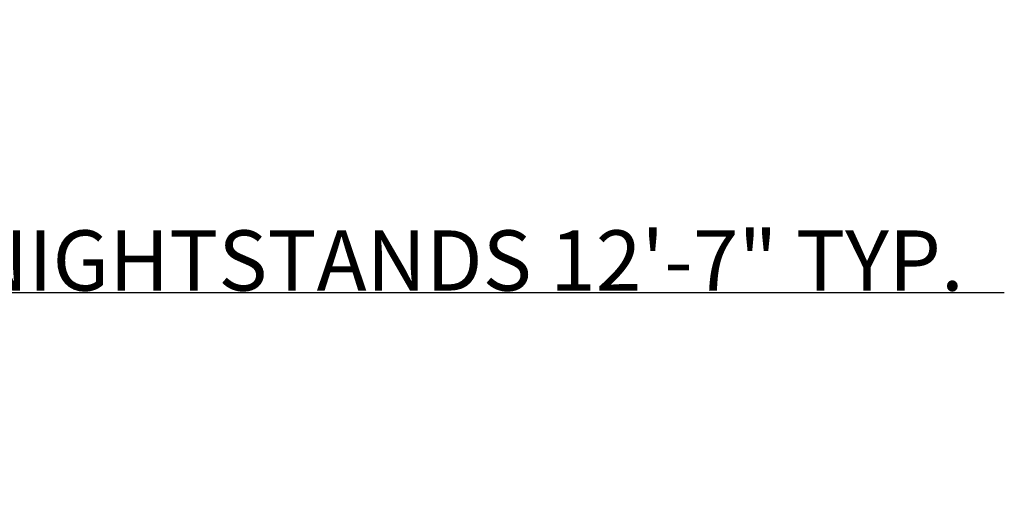
# Model space of a CAD drawing. Units: inches. Extents: x 351 to 1738, y -265 to 286.
# Tile 38 of 38: x 1607 to 1738, y 22 to 86. Entities that reach past the tile are written whole.
import ezdxf

# ---------------------------------------------------------------- set-up
doc = ezdxf.new("R2010")
doc.units = ezdxf.units.IN
doc.header["$MEASUREMENT"] = 0
doc.layers.add('A-ANNO-DIMS', color=2, linetype='Continuous', lineweight=18)
doc.styles.get("Standard").update_dxf_attribs({"font": 'arial.ttf'})
doc.dimstyles.get("Standard").update_dxf_attribs({"dimtxt": 8, "dimasz": 5, "dimexe": 0.18, "dimexo": 0.0625, "dimgap": 0.09, "dimtad": 1, "dimtoh": 1, "dimzin": 0, "dimdsep": 46, "dimlunit": 4, "dimtxsty": 'Standard', "dimcen": 0, "dimclre": 256, "dimadec": 0, "dimazin": 0, "dimtfac": 1, "dimtofl": 0, "dimtmove": 0, "dimatfit": 3, "dimfxl": 1, "dimtolj": 1, "dimtzin": 0, "dimlwe": -1, "dimarcsym": 0})

# ---------------------------------------------------------------- blocks, each defined once
blk = doc.blocks.new('*D46')
at = {"layer": 'A-ANNO-DIMS', "transparency": 16777216}
for p, q in [((1391.39, 72.13), (1391.39, 49.37)), ((1542.29, 72.13), (1542.29, 49.37))]:
    blk.add_line(p, q, dxfattribs=at)
at = {"layer": 'A-ANNO-DIMS', "color": 0, "lineweight": -2, "transparency": 16777216}
for p, q in [((1396.39, 49.55), (1537.29, 49.55)), ((1542.29, 49.55), (1738.09, 49.55))]:
    blk.add_line(p, q, dxfattribs=at)
at = {"layer": 'A-ANNO-DIMS', "color": 0, "transparency": 16777216}
for points in [[(1396.39, 50.39), (1396.39, 48.72), (1391.39, 49.55)], [(1537.29, 50.39), (1537.29, 48.72), (1542.29, 49.55)]]:
    blk.add_solid(points, dxfattribs=at)
at = {"layer": 'Defpoints', "color": 0, "transparency": 16777216}
for p in [(1391.39, 72.19), (1542.29, 72.19), (1542.29, 49.55)]:
    blk.add_point(p, dxfattribs=at)
at = {"layer": 'A-ANNO-DIMS', "color": 0, "transparency": 16777216, "insert": (1642.69, 53.78), "char_height": 8, "attachment_point": 5}
blk.add_mtext('\\A1;BED AND NIGHTSTANDS 12\'-7" TYP.', dxfattribs=at)

msp = doc.modelspace()

# ---------------------------------------------------------------- dimensions: what is measured, and where the dimension line sits
at = {"layer": 'A-ANNO-DIMS'}
dim = msp.add_linear_dim(base=(1542.294, 49.553), p1=(1391.393, 72.188), p2=(1542.294, 72.188), text='BED AND NIGHTSTANDS <> TYP.', dimstyle='Standard', override={"dimdec": 1, "dimlfac": 1, "dimrnd": 0, "dimzin": 1, "dimdsep": 46, "dimlunit": 4, "dimfrac": 2}, dxfattribs=at)
dim.commit()
dim.dimension.update_dxf_attribs({"geometry": '*D46', "text_midpoint": (1642.691, 53.779)})

doc.saveas('drawing.dxf')
